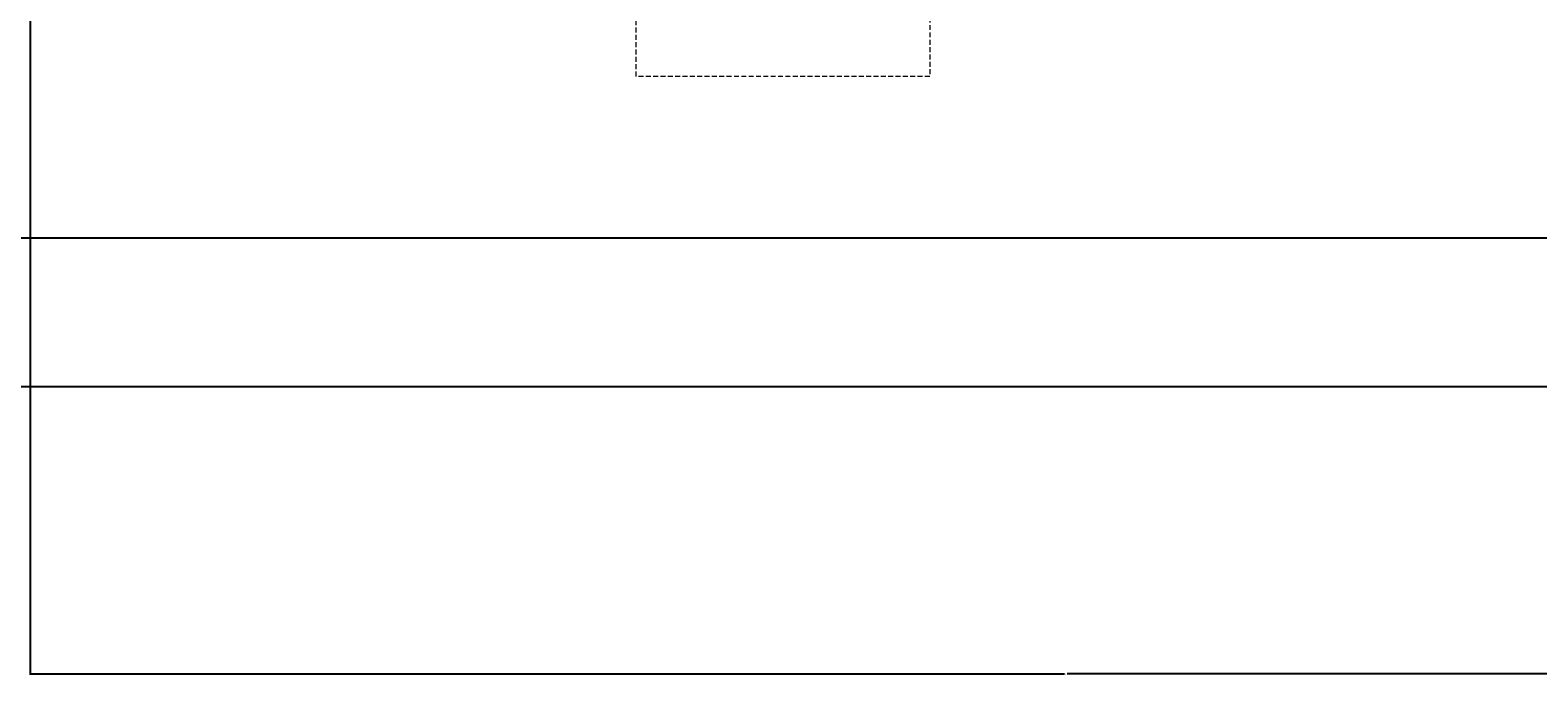
# Model space of a CAD drawing. Units: inches. Extents: x 1693 to 2974, y 2201 to 2965.
# Tile 16 of 24: x 2479 to 2787, y 2201 to 2332. Entities that reach past the tile are written whole.
import ezdxf

# ---------------------------------------------------------------- set-up
doc = ezdxf.new("R2010")
doc.units = ezdxf.units.IN
doc.header["$LTSCALE"] = 2
doc.header["$MEASUREMENT"] = 0
doc.linetypes.add('HIDDEN', pattern=[0.375, 0.25, -0.125])
doc.layers.add('A-ANNO-DIMS', color=2, linetype='Continuous', lineweight=18)
doc.layers.add('A-GLAZ-OVHD', color=8, linetype='HIDDEN', lineweight=13)
doc.styles.get("Standard").update_dxf_attribs({"font": 'arial.ttf'})
doc.dimstyles.get("Standard").update_dxf_attribs({"dimtxt": 0.18, "dimasz": 0.18, "dimexe": 0.18, "dimexo": 0.0625, "dimgap": 0.09, "dimtad": 0, "dimtih": 1, "dimtoh": 1, "dimdec": 1, "dimzin": 0, "dimdsep": 46, "dimlunit": 3, "dimtxsty": 'Standard', "dimcen": 0.09, "dimadec": 0, "dimazin": 0, "dimtfac": 1, "dimtdec": 1, "dimtofl": 0, "dimtmove": 0, "dimatfit": 3, "dimfxl": 1, "dimtolj": 1, "dimtzin": 0, "dimarcsym": 0})

# ---------------------------------------------------------------- blocks, each defined once
blk = doc.blocks.new('*D82')
at = {"layer": 'A-ANNO-DIMS', "color": 0, "lineweight": -2, "ltscale": 2, "transparency": 16777216}
for p, q in [((2615.67, 2906.08), (1693.46, 2906.08)), ((1693.64, 2905.9), (1693.64, 2582.94)), ((1693.64, 2259.62), (1693.64, 2582.58)), ((2096.17, 2259.44), (1693.46, 2259.44))]:
    blk.add_line(p, q, dxfattribs=at)
at = {"layer": 'A-ANNO-DIMS', "color": 0, "ltscale": 2, "transparency": 16777216}
for points in [[(1693.61, 2905.9), (1693.67, 2905.9), (1693.64, 2906.08)], [(1693.61, 2259.62), (1693.67, 2259.62), (1693.64, 2259.44)]]:
    blk.add_solid(points, dxfattribs=at)
at = {"layer": 'Defpoints', "color": 0, "ltscale": 2, "transparency": 16777216}
for p in [(1693.64, 2906.08), (2615.74, 2906.08), (2096.24, 2259.44)]:
    blk.add_point(p, dxfattribs=at)
at = {"layer": 'A-ANNO-DIMS', "color": 0, "ltscale": 2, "transparency": 16777216, "insert": (1693.64, 2582.76), "char_height": 0.18, "attachment_point": 5}
blk.add_mtext('\\A1;646.6', dxfattribs=at)
blk = doc.blocks.new('*D85')
at = {"layer": 'A-ANNO-DIMS', "color": 0, "lineweight": -2, "ltscale": 2, "transparency": 16777216}
for p, q in [((2479.24, 2334.69), (2479.24, 2200.56)), ((2902.24, 2334.69), (2902.24, 2200.56)), ((2479.42, 2200.74), (2690.44, 2200.74)), ((2902.06, 2200.74), (2691.03, 2200.74))]:
    blk.add_line(p, q, dxfattribs=at)
at = {"layer": 'A-ANNO-DIMS', "color": 0, "ltscale": 2, "transparency": 16777216}
for points in [[(2479.42, 2200.77), (2479.42, 2200.71), (2479.24, 2200.74)], [(2902.06, 2200.77), (2902.06, 2200.71), (2902.24, 2200.74)]]:
    blk.add_solid(points, dxfattribs=at)
at = {"layer": 'Defpoints', "color": 0, "ltscale": 2, "transparency": 16777216}
for p in [(2479.24, 2334.75), (2902.24, 2334.75), (2902.24, 2200.74)]:
    blk.add_point(p, dxfattribs=at)
at = {"layer": 'A-ANNO-DIMS', "color": 0, "ltscale": 2, "transparency": 16777216, "insert": (2690.74, 2200.74), "char_height": 0.18, "attachment_point": 5}
blk.add_mtext('\\A1;423', dxfattribs=at)
blk = doc.blocks.new('*D89')
at = {"layer": 'A-ANNO-DIMS', "color": 0, "lineweight": -2, "ltscale": 2, "transparency": 16777216}
for p, q in [((2479.3, 2334.75), (2973.12, 2334.75)), ((2972.94, 2334.57), (2972.94, 2312.48)), ((2972.94, 2290.02), (2972.94, 2312.12)), ((2294.3, 2289.84), (2973.12, 2289.84))]:
    blk.add_line(p, q, dxfattribs=at)
at = {"layer": 'A-ANNO-DIMS', "color": 0, "ltscale": 2, "transparency": 16777216}
for points in [[(2972.91, 2334.57), (2972.97, 2334.57), (2972.94, 2334.75)], [(2972.91, 2290.02), (2972.97, 2290.02), (2972.94, 2289.84)]]:
    blk.add_solid(points, dxfattribs=at)
at = {"layer": 'Defpoints', "color": 0, "ltscale": 2, "transparency": 16777216}
for p in [(2479.24, 2334.75), (2972.94, 2334.75), (2294.24, 2289.84)]:
    blk.add_point(p, dxfattribs=at)
at = {"layer": 'A-ANNO-DIMS', "color": 0, "ltscale": 2, "transparency": 16777216, "insert": (2972.94, 2312.3), "char_height": 0.18, "attachment_point": 5}
blk.add_mtext('\\A1;44.91', dxfattribs=at)
blk = doc.blocks.new('*D95')
at = {"layer": 'A-ANNO-DIMS', "color": 0, "lineweight": -2, "ltscale": 2, "transparency": 16777216}
for p, q in [((2189.3, 2289.84), (2973.12, 2289.84)), ((2972.94, 2289.66), (2972.94, 2274.83)), ((2972.94, 2259.62), (2972.94, 2274.46)), ((2189.3, 2259.44), (2973.12, 2259.44))]:
    blk.add_line(p, q, dxfattribs=at)
at = {"layer": 'A-ANNO-DIMS', "color": 0, "ltscale": 2, "transparency": 16777216}
for points in [[(2972.91, 2289.66), (2972.97, 2289.66), (2972.94, 2289.84)], [(2972.91, 2259.62), (2972.97, 2259.62), (2972.94, 2259.44)]]:
    blk.add_solid(points, dxfattribs=at)
at = {"layer": 'Defpoints', "color": 0, "ltscale": 2, "transparency": 16777216}
for p in [(2189.24, 2289.84), (2972.94, 2289.84), (2189.24, 2259.44)]:
    blk.add_point(p, dxfattribs=at)
at = {"layer": 'A-ANNO-DIMS', "color": 0, "ltscale": 2, "transparency": 16777216, "insert": (2972.94, 2274.64), "char_height": 0.18, "attachment_point": 5}
blk.add_mtext('\\A1;30.4', dxfattribs=at)

msp = doc.modelspace()

# ---------------------------------------------------------------- linework, layer by layer
at = {"layer": 'A-GLAZ-OVHD', "ltscale": 2}
for p, q in [((2602.9702, 2322.7547), (2602.9702, 2334.7547)), ((2662.9702, 2334.7547), (2662.9702, 2322.7547)), ((2608.9702, 2322.7547), (2602.9702, 2322.7547)), ((2662.9702, 2322.7547), (2608.9702, 2322.7547))]:
    msp.add_line(p, q, dxfattribs=at)

# ---------------------------------------------------------------- dimensions: what is measured, and where the dimension line sits
at = {"layer": 'A-ANNO-DIMS', "ltscale": 2}
for base, p1, p2, override, picture, middle in [((1693.6363, 2906.0761), (2096.2363, 2259.4449), (2615.7363, 2906.0761), {"dimdec": 1, "dimlfac": 1, "dimrnd": 0, "dimzin": 0, "dimdsep": 46, "dimlunit": 2}, '*D82', (1693.6363, 2582.7605)), ((2972.9363, 2334.7547), (2294.2363, 2289.8449), (2479.2363, 2334.7547), {"dimdec": 2, "dimlfac": 1, "dimrnd": 0, "dimzin": 0, "dimdsep": 46, "dimlunit": 2}, '*D89', (2972.9363, 2312.2998)), ((2972.9363, 2289.8449), (2189.2363, 2259.4449), (2189.2363, 2289.8449), {"dimdec": 1, "dimlfac": 1, "dimrnd": 0, "dimzin": 0, "dimdsep": 46, "dimlunit": 2}, '*D95', (2972.9363, 2274.6449))]:
    dim = msp.add_linear_dim(base=base, p1=p1, p2=p2, angle=90, dimstyle='Standard', override=override, dxfattribs=at)
    dim.commit()
    dim.dimension.update_dxf_attribs({"geometry": picture, "text_midpoint": middle})
dim = msp.add_linear_dim(base=(2902.2363, 2200.7449), p1=(2479.2363, 2334.7547), p2=(2902.2363, 2334.7547), dimstyle='Standard', override={"dimdec": 0, "dimlfac": 1, "dimrnd": 0, "dimzin": 0, "dimdsep": 46, "dimlunit": 2}, dxfattribs=at)
dim.commit()
dim.dimension.update_dxf_attribs({"geometry": '*D85', "text_midpoint": (2690.7363, 2200.7449)})

doc.saveas('drawing.dxf')
